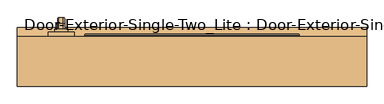
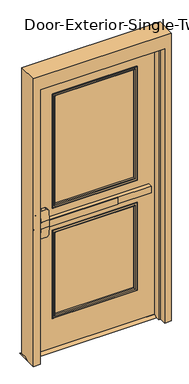
"""IFC4 building model written with IfcOpenShell, lengths in millimetres: door geometry, Door-Exterior-Single-Two_Lite : Door-Exterior-Single-Two_Lite."""

from ifc_helpers import new_model, si_unit, point, frame, frame_2d, origin, place, context, project, spatial, polyline, circle_curve, ellipse_curve, trimmed, segment, composite_curve, outline, extrude, faceted_brep, source, transform, mapped, element, save
from ifc_brep_helpers import plane_surface, cylinder_surface, revolved_surface, advanced_brep


def door_exterior_single_two_lite_door_exterior_single_two_lite_fa13afaf(model_context):
    return source(origin(), model_context, "Body", "SolidModel", [
        extrude(outline(polyline([(44.0, 12.7), (88.45, 12.7), (113.85, 0.0), (18.6, 0.0), (44.0, 12.7)])), frame((-508.0, 0.0, 0.0), z_axis=(1.0, 0.0, 0.0), x_axis=(0.0, 1.0, 0.0)), (0.0, 0.0, 1.0), 1016.0),
        extrude(outline(polyline([(150.2833333, 5.9), (-349.25, 5.9), (-349.25, 12.25), (150.2833333, 12.25), (150.2833333, 5.9)])), frame((0.0, 0.0, 990.6), z_axis=(0.0, 0.0, 1.0), x_axis=(1.0, 0.0, 0.0)), (0.0, 0.0, 1.0), 50.8),
        advanced_brep(
        [(-412.75, 12.25, 1041.4), (-412.75, 12.25, 990.6), (-349.25, 12.25, 990.6), (400.05, 12.25, 990.6), (400.05, 12.25, 1041.4), (-349.25, 12.25, 1041.4), (400.05, 44.0, 1041.4), (400.05, 44.0, 990.6), (-349.25, 44.0, 990.6), (-349.25, 44.0, 927.1), (-368.3, 44.0, 908.05), (-393.7, 44.0, 908.05), (-412.75, 44.0, 927.1), (-412.75, 44.0, 1104.9), (-393.7, 44.0, 1123.95), (-368.3, 44.0, 1123.95), (-349.25, 44.0, 1104.9), (-349.25, 44.0, 1041.4), (-349.25, 15.4252467, 1041.4), (-412.75, 15.4252467, 1041.4), (-412.75, 20.4354269, 1104.9), (-412.75, 20.4354269, 927.1), (-412.75, 15.4252467, 990.6), (-349.25, 15.4252467, 990.6), (-349.25, 20.4354269, 927.1), (-349.25, 20.4354269, 1104.9), (-393.7, 21.938481, 1123.95), (-368.3, 21.938481, 1123.95), (-368.3, 21.938481, 908.05), (-393.7, 21.938481, 908.05)],
        [
            (0, 1),
            (1, 2),
            (2, 3),
            (3, 4),
            (4, 5),
            (5, 0),
            (6, 7),
            (7, 8),
            (8, 9),
            (9, 10, circle_curve(frame((-368.3, 44.0, 927.1), z_axis=(0.0, 1.0, 0.0), x_axis=(1.0, 0.0, 0.0)), 19.05)),
            (10, 11),
            (11, 12, circle_curve(frame((-393.7, 44.0, 927.1), z_axis=(0.0, 1.0, 0.0), x_axis=(1.0, 0.0, 0.0)), 19.05)),
            (12, 13),
            (13, 14, circle_curve(frame((-393.7, 44.0, 1104.9), z_axis=(0.0, 1.0, 0.0), x_axis=(1.0, 0.0, 0.0)), 19.05)),
            (14, 15),
            (15, 16, circle_curve(frame((-368.3, 44.0, 1104.9), z_axis=(0.0, 1.0, 0.0), x_axis=(1.0, 0.0, 0.0)), 19.05)),
            (16, 17),
            (17, 6),
            (4, 6),
            (17, 18),
            (18, 19),
            (19, 0),
            (19, 20),
            (20, 13),
            (12, 21),
            (21, 22),
            (22, 1),
            (7, 3),
            (22, 23),
            (23, 8),
            (23, 24),
            (24, 9),
            (16, 25),
            (25, 18),
            (14, 26),
            (26, 27),
            (27, 15),
            (10, 28),
            (28, 29),
            (29, 11),
            (24, 28, ellipse_curve(frame((-368.3, 20.4354269, 927.1), z_axis=(0.0, 0.9969018152893365, 0.07865602756830282), x_axis=(0.0, -0.07865602756830208, 0.9969018152893365)), 19.1092038, 19.05)),
            (27, 25, ellipse_curve(frame((-368.3, 20.4354269, 1104.9), z_axis=(0.0, 0.9969018152893376, -0.07865602756828934), x_axis=(0.0, -0.078656027568288, -0.9969018152893377)), 19.1092038, 19.05)),
            (20, 26, ellipse_curve(frame((-393.7, 20.4354269, 1104.9), z_axis=(0.0, 0.9969018152893376, -0.07865602756828934), x_axis=(0.0, -0.078656027568288, -0.9969018152893377)), 19.1092038, 19.05)),
            (29, 21, ellipse_curve(frame((-393.7, 20.4354269, 927.1), z_axis=(0.0, 0.9969018152893365, 0.07865602756830282), x_axis=(0.0, -0.07865602756830208, 0.9969018152893365)), 19.1092038, 19.05)),
        ],
        [
            plane_surface(frame((-412.75, 12.25, 1041.4), z_axis=(0.0, -1.0, 0.0), x_axis=(-1.0, 0.0, 0.0))),
            plane_surface(frame((-412.75, 44.0, 1041.4), z_axis=(0.0, 1.0, 0.0), x_axis=(1.0, 0.0, 0.0))),
            plane_surface(frame((400.05, 12.25, 1041.4), z_axis=(0.0, 0.0, 1.0), x_axis=(0.0, 1.0, 0.0))),
            plane_surface(frame((-412.75, 12.25, 1041.4), z_axis=(-1.0, 0.0, 0.0), x_axis=(0.0, 1.0, 0.0))),
            plane_surface(frame((-412.75, 12.25, 990.6), z_axis=(0.0, 0.0, -1.0), x_axis=(0.0, 1.0, 0.0))),
            plane_surface(frame((400.05, 12.25, 990.6), z_axis=(1.0, 0.0, 0.0), x_axis=(0.0, 1.0, 0.0))),
            plane_surface(frame((-349.25, 15.4252467, 927.1), z_axis=(1.0, 0.0, 0.0), x_axis=(0.0, 1.0, 0.0))),
            plane_surface(frame((-368.3, 15.4252467, 1123.95), z_axis=(0.0, 0.0, 1.0), x_axis=(0.0, 1.0, 0.0))),
            plane_surface(frame((-393.7, 15.4252467, 908.05), z_axis=(0.0, 0.0, -1.0), x_axis=(0.0, 1.0, 0.0))),
            cylinder_surface(frame((-368.3, 44.0, 927.1), z_axis=(0.0, -1.0, 0.0), x_axis=(1.0, 0.0, 0.0)), 19.05),
            cylinder_surface(frame((-368.3, 44.0, 1104.9), z_axis=(0.0, -1.0, 0.0), x_axis=(1.0, 0.0, 0.0)), 19.05),
            cylinder_surface(frame((-393.7, 44.0, 1104.9), z_axis=(0.0, -1.0, 0.0), x_axis=(1.0, 0.0, 0.0)), 19.05),
            cylinder_surface(frame((-393.7, 44.0, 927.1), z_axis=(0.0, -1.0, 0.0), x_axis=(1.0, 0.0, 0.0)), 19.05),
            plane_surface(frame((-349.25, 15.4252467, 1041.4), z_axis=(0.0, -0.9969018152893376, 0.07865602756828934), x_axis=(-1.0, 0.0, 0.0))),
            plane_surface(frame((-349.25, 21.938481, 908.05), z_axis=(0.0, -0.9969018152893365, -0.07865602756830282), x_axis=(-1.0, 0.0, 0.0))),
        ],
        [
            (0, [[1, 2, 3, 4, 5, 6]]),
            (1, [[7, 8, 9, 10, 11, 12, 13, 14, 15, 16, 17, 18]]),
            (2, [[19, -18, 20, 21, 22, -6, -5]]),
            (3, [[-1, -22, 23, 24, -13, 25, 26, 27]]),
            (4, [[28, -3, -2, -27, 29, 30, -8]]),
            (5, [[-4, -28, -7, -19]]),
            (6, [[-9, -30, 31, 32]]),
            (6, [[-17, 33, 34, -20]]),
            (7, [[-15, 35, 36, 37]]),
            (8, [[-11, 38, 39, 40]]),
            (9, [[-10, -32, 41, -38]]),
            (10, [[-16, -37, 42, -33]]),
            (11, [[-14, -24, 43, -35]]),
            (12, [[-12, -40, 44, -25]]),
            (13, [[-21, -34, -42, -36, -43, -23]]),
            (14, [[-26, -44, -39, -41, -31, -29]]),
        ],
    ),
        advanced_brep(
        [(-391.0, 101.15, 1017.190625), (-391.0, 101.15, 1014.809375), (-387.428125, 101.15, 1011.2375), (-374.5715406, 101.15, 1011.2375), (-371.0, 101.15, 1014.8090406), (-371.0, 101.15, 1017.190625), (-374.571875, 101.15, 1020.7625), (-387.428125, 101.15, 1020.7625), (-391.0, 101.15, 887.809375), (-387.428125, 101.15, 884.2375), (-374.571875, 101.15, 884.2375), (-371.0, 101.15, 887.809375), (-371.0, 101.15, 890.1909594), (-374.5715406, 101.15, 893.7625), (-387.428125, 101.15, 893.7625), (-391.0, 101.15, 890.190625), (-391.0, 126.55, 1017.190625), (-391.0, 140.440625, 1003.3), (-391.0, 140.440625, 901.7), (-391.0, 126.55, 887.809375), (-391.0, 126.55, 890.190625), (-391.0, 138.059375, 901.7), (-391.0, 138.059375, 1003.3), (-391.0, 126.55, 1014.809375), (-387.428125, 126.55, 1011.2375), (-374.5715406, 126.55, 1011.2375), (-371.0, 126.55, 1014.8090406), (-371.0, 138.0590406, 1003.3), (-371.0, 138.0590406, 901.7), (-371.0, 126.55, 890.1909594), (-371.0, 126.55, 887.809375), (-371.0, 140.440625, 901.7), (-371.0, 140.440625, 1003.3), (-371.0, 126.55, 1017.190625), (-374.571875, 126.55, 1020.7625), (-387.428125, 126.55, 1020.7625), (-387.428125, 134.4875, 1003.3), (-374.5715406, 134.4875, 1003.3), (-374.571875, 144.0125, 1003.3), (-387.428125, 144.0125, 1003.3), (-387.428125, 134.4875, 901.7), (-374.5715406, 134.4875, 901.7), (-374.571875, 144.0125, 901.7), (-387.428125, 144.0125, 901.7), (-387.428125, 126.55, 893.7625), (-374.5715406, 126.55, 893.7625), (-374.571875, 126.55, 884.2375), (-387.428125, 126.55, 884.2375)],
        [
            (0, 1),
            (1, 2, circle_curve(frame((-387.428125, 101.15, 1014.809375), z_axis=(0.0, -1.0, 0.0), x_axis=(0.0, 0.0, 1.0)), 3.571875)),
            (2, 3),
            (3, 4, circle_curve(frame((-374.5715406, 101.15, 1014.8090406), z_axis=(0.0, -1.0, 0.0), x_axis=(0.0, 0.0, 1.0)), 3.5715406)),
            (4, 5),
            (5, 6, circle_curve(frame((-374.571875, 101.15, 1017.190625), z_axis=(0.0, -1.0, 0.0), x_axis=(0.0, 0.0, 1.0)), 3.571875)),
            (6, 7),
            (7, 0, circle_curve(frame((-387.428125, 101.15, 1017.190625), z_axis=(0.0, -1.0, 0.0), x_axis=(0.0, 0.0, 1.0)), 3.571875)),
            (8, 9, circle_curve(frame((-387.428125, 101.15, 887.809375), z_axis=(0.0, -1.0, 0.0), x_axis=(0.0, 0.0, -1.0)), 3.571875)),
            (9, 10),
            (10, 11, circle_curve(frame((-374.571875, 101.15, 887.809375), z_axis=(0.0, -1.0, 0.0), x_axis=(0.0, 0.0, -1.0)), 3.571875)),
            (11, 12),
            (12, 13, circle_curve(frame((-374.5715406, 101.15, 890.1909594), z_axis=(0.0, -1.0, 0.0), x_axis=(0.0, 0.0, -1.0)), 3.5715406)),
            (13, 14),
            (14, 15, circle_curve(frame((-387.428125, 101.15, 890.190625), z_axis=(0.0, -1.0, 0.0), x_axis=(0.0, 0.0, -1.0)), 3.571875)),
            (15, 8),
            (0, 16),
            (16, 17, circle_curve(frame((-391.0, 126.55, 1003.3), z_axis=(-1.0, 0.0, 0.0), x_axis=(0.0, 0.0, 1.0)), 13.890625)),
            (17, 18),
            (18, 19, circle_curve(frame((-391.0, 126.55, 901.7), z_axis=(-1.0, 0.0, 0.0), x_axis=(0.0, 1.0, 0.0)), 13.890625)),
            (19, 8),
            (15, 20),
            (20, 21, circle_curve(frame((-391.0, 126.55, 901.7), z_axis=(1.0, 0.0, 0.0), x_axis=(0.0, 1.0, 0.0)), 11.509375)),
            (21, 22),
            (22, 23, circle_curve(frame((-391.0, 126.55, 1003.3), z_axis=(1.0, 0.0, 0.0), x_axis=(0.0, 0.0, 1.0)), 11.509375)),
            (23, 1),
            (23, 24, circle_curve(frame((-387.428125, 126.55, 1014.809375), z_axis=(0.0, -1.0, 0.0), x_axis=(0.0, 0.0, 1.0)), 3.571875)),
            (24, 2),
            (24, 25),
            (25, 3),
            (25, 26, circle_curve(frame((-374.5715406, 126.55, 1014.8090406), z_axis=(0.0, -1.0, 0.0), x_axis=(0.0, 0.0, 1.0)), 3.5715406)),
            (26, 4),
            (26, 27, circle_curve(frame((-371.0, 126.55, 1003.3), z_axis=(-1.0, 0.0, 0.0), x_axis=(0.0, 0.0, 1.0)), 11.5090406)),
            (27, 28),
            (28, 29, circle_curve(frame((-371.0, 126.55, 901.7), z_axis=(-1.0, 0.0, 0.0), x_axis=(0.0, 1.0, 0.0)), 11.5090406)),
            (29, 12),
            (11, 30),
            (30, 31, circle_curve(frame((-371.0, 126.55, 901.7), z_axis=(1.0, 0.0, 0.0), x_axis=(0.0, 1.0, 0.0)), 13.890625)),
            (31, 32),
            (32, 33, circle_curve(frame((-371.0, 126.55, 1003.3), z_axis=(1.0, 0.0, 0.0), x_axis=(0.0, 0.0, 1.0)), 13.890625)),
            (33, 5),
            (33, 34, circle_curve(frame((-374.571875, 126.55, 1017.190625), z_axis=(0.0, -1.0, 0.0), x_axis=(0.0, 0.0, 1.0)), 3.571875)),
            (34, 6),
            (34, 35),
            (35, 7),
            (35, 16, circle_curve(frame((-387.428125, 126.55, 1017.190625), z_axis=(0.0, -1.0, 0.0), x_axis=(0.0, 0.0, 1.0)), 3.571875)),
            (36, 24, circle_curve(frame((-387.428125, 126.55, 1003.3), z_axis=(1.0, 0.0, 0.0), x_axis=(0.0, 0.0, 1.0)), 7.9375)),
            (22, 36, circle_curve(frame((-387.428125, 138.059375, 1003.3), z_axis=(0.0, 0.0, 1.0), x_axis=(0.0, 1.0, 0.0)), 3.571875)),
            (37, 25, circle_curve(frame((-374.5715406, 126.55, 1003.3), z_axis=(1.0, 0.0, 0.0), x_axis=(0.0, 0.0, 1.0)), 7.9375)),
            (36, 37),
            (37, 27, circle_curve(frame((-374.5715406, 138.0590406, 1003.3), z_axis=(0.0, 0.0, 1.0), x_axis=(0.0, 1.0, 0.0)), 3.5715406)),
            (38, 34, circle_curve(frame((-374.571875, 126.55, 1003.3), z_axis=(1.0, 0.0, 0.0), x_axis=(0.0, 0.0, 1.0)), 17.4625)),
            (32, 38, circle_curve(frame((-374.571875, 140.440625, 1003.3), z_axis=(0.0, 0.0, 1.0), x_axis=(0.0, 1.0, 0.0)), 3.571875)),
            (39, 35, circle_curve(frame((-387.428125, 126.55, 1003.3), z_axis=(1.0, 0.0, 0.0), x_axis=(0.0, 0.0, 1.0)), 17.4625)),
            (38, 39),
            (39, 17, circle_curve(frame((-387.428125, 140.440625, 1003.3), z_axis=(0.0, 0.0, 1.0), x_axis=(0.0, 1.0, 0.0)), 3.571875)),
            (21, 40, circle_curve(frame((-387.428125, 138.059375, 901.7), z_axis=(0.0, 0.0, 1.0), x_axis=(0.0, 1.0, 0.0)), 3.571875)),
            (40, 36),
            (40, 41),
            (41, 37),
            (41, 28, circle_curve(frame((-374.5715406, 138.0590406, 901.7), z_axis=(0.0, 0.0, 1.0), x_axis=(0.0, 1.0, 0.0)), 3.5715406)),
            (31, 42, circle_curve(frame((-374.571875, 140.440625, 901.7), z_axis=(0.0, 0.0, 1.0), x_axis=(0.0, 1.0, 0.0)), 3.571875)),
            (42, 38),
            (42, 43),
            (43, 39),
            (43, 18, circle_curve(frame((-387.428125, 140.440625, 901.7), z_axis=(0.0, 0.0, 1.0), x_axis=(0.0, 1.0, 0.0)), 3.571875)),
            (44, 40, circle_curve(frame((-387.428125, 126.55, 901.7), z_axis=(1.0, 0.0, 0.0), x_axis=(0.0, 1.0, 0.0)), 7.9375)),
            (20, 44, circle_curve(frame((-387.428125, 126.55, 890.190625), z_axis=(0.0, 1.0, 0.0), x_axis=(0.0, 0.0, -1.0)), 3.571875)),
            (45, 41, circle_curve(frame((-374.5715406, 126.55, 901.7), z_axis=(1.0, 0.0, 0.0), x_axis=(0.0, 1.0, 0.0)), 7.9375)),
            (44, 45),
            (45, 29, circle_curve(frame((-374.5715406, 126.55, 890.1909594), z_axis=(0.0, 1.0, 0.0), x_axis=(0.0, 0.0, -1.0)), 3.5715406)),
            (46, 42, circle_curve(frame((-374.571875, 126.55, 901.7), z_axis=(1.0, 0.0, 0.0), x_axis=(0.0, 1.0, 0.0)), 17.4625)),
            (30, 46, circle_curve(frame((-374.571875, 126.55, 887.809375), z_axis=(0.0, 1.0, 0.0), x_axis=(0.0, 0.0, -1.0)), 3.571875)),
            (47, 43, circle_curve(frame((-387.428125, 126.55, 901.7), z_axis=(1.0, 0.0, 0.0), x_axis=(0.0, 1.0, 0.0)), 17.4625)),
            (46, 47),
            (47, 19, circle_curve(frame((-387.428125, 126.55, 887.809375), z_axis=(0.0, 1.0, 0.0), x_axis=(0.0, 0.0, -1.0)), 3.571875)),
            (14, 44),
            (13, 45),
            (10, 46),
            (9, 47),
        ],
        [
            plane_surface(frame((-381.0, 101.15, 1016.0), z_axis=(0.0, -1.0, 0.0), x_axis=(1.0, 0.0, 0.0))),
            plane_surface(frame((-381.0, 101.15, 889.0), z_axis=(0.0, -1.0, 0.0), x_axis=(1.0, 0.0, 0.0))),
            plane_surface(frame((-391.0, 101.15, 1017.190625), z_axis=(-1.0, 0.0, 0.0), x_axis=(0.0, 1.0, 0.0))),
            cylinder_surface(frame((-387.428125, 101.15, 1014.809375), z_axis=(0.0, -1.0, 0.0), x_axis=(0.0, 0.0, 1.0)), 3.571875),
            plane_surface(frame((-387.428125, 101.15, 1011.2375), z_axis=(0.0, 0.0, -1.0), x_axis=(0.0, 1.0, 0.0))),
            cylinder_surface(frame((-374.5715406, 101.15, 1014.8090406), z_axis=(0.0, -1.0, 0.0), x_axis=(0.0, 0.0, 1.0)), 3.5715406),
            plane_surface(frame((-371.0, 101.15, 1014.8090406), z_axis=(1.0, 0.0, 0.0), x_axis=(0.0, 1.0, 0.0))),
            cylinder_surface(frame((-374.571875, 101.15, 1017.190625), z_axis=(0.0, -1.0, 0.0), x_axis=(0.0, 0.0, 1.0)), 3.571875),
            plane_surface(frame((-374.571875, 101.15, 1020.7625), z_axis=(0.0, 0.0, 1.0), x_axis=(0.0, 1.0, 0.0))),
            cylinder_surface(frame((-387.428125, 101.15, 1017.190625), z_axis=(0.0, -1.0, 0.0), x_axis=(0.0, 0.0, 1.0)), 3.571875),
            revolved_surface(trimmed(ellipse_curve(frame((-387.428125, 126.55, 1014.809375), z_axis=(0.0, -1.0, 0.0), x_axis=(0.0, 0.0, 1.0)), 3.571875, 3.571875), [point((-391.0, 126.55, 1014.809375))], [point((-387.428125, 126.55, 1011.2375))], True, "CARTESIAN"), (-381.0, 126.55, 1003.3), (-1.0, 0.0, 0.0)),
            revolved_surface(polyline([(-387.428125, 126.55, 1011.2375), (-374.5715406, 126.55, 1011.2375)]), (-381.0, 126.55, 1003.3), (-1.0, 0.0, 0.0)),
            revolved_surface(trimmed(ellipse_curve(frame((-374.5715406, 126.55, 1014.8090406), z_axis=(0.0, -1.0, 0.0), x_axis=(0.0, 0.0, 1.0)), 3.5715406, 3.5715406), [point((-374.5715406, 126.55, 1011.2375))], [point((-371.0, 126.55, 1014.8090406))], True, "CARTESIAN"), (-381.0, 126.55, 1003.3), (-1.0, 0.0, 0.0)),
            revolved_surface(trimmed(ellipse_curve(frame((-374.571875, 126.55, 1017.190625), z_axis=(0.0, -1.0, 0.0), x_axis=(0.0, 0.0, 1.0)), 3.571875, 3.571875), [point((-371.0, 126.55, 1017.190625))], [point((-374.571875, 126.55, 1020.7625))], True, "CARTESIAN"), (-381.0, 126.55, 1003.3), (-1.0, 0.0, 0.0)),
            cylinder_surface(frame((-381.0, 126.55, 1003.3), z_axis=(-1.0, 0.0, 0.0), x_axis=(0.0, 0.0, 1.0)), 17.4625),
            revolved_surface(trimmed(ellipse_curve(frame((-387.428125, 126.55, 1017.190625), z_axis=(0.0, -1.0, 0.0), x_axis=(0.0, 0.0, 1.0)), 3.571875, 3.571875), [point((-387.428125, 126.55, 1020.7625))], [point((-391.0, 126.55, 1017.190625))], True, "CARTESIAN"), (-381.0, 126.55, 1003.3), (-1.0, 0.0, 0.0)),
            cylinder_surface(frame((-387.428125, 138.059375, 1003.3), z_axis=(0.0, 0.0, 1.0), x_axis=(0.0, 1.0, 0.0)), 3.571875),
            plane_surface(frame((-387.428125, 134.4875, 1003.3), z_axis=(0.0, -1.0, 0.0), x_axis=(0.0, 0.0, -1.0))),
            cylinder_surface(frame((-374.5715406, 138.0590406, 1003.3), z_axis=(0.0, 0.0, 1.0), x_axis=(0.0, 1.0, 0.0)), 3.5715406),
            cylinder_surface(frame((-374.571875, 140.440625, 1003.3), z_axis=(0.0, 0.0, 1.0), x_axis=(0.0, 1.0, 0.0)), 3.571875),
            plane_surface(frame((-374.571875, 144.0125, 1003.3), z_axis=(0.0, 1.0, 0.0), x_axis=(0.0, 0.0, -1.0))),
            cylinder_surface(frame((-387.428125, 140.440625, 1003.3), z_axis=(0.0, 0.0, 1.0), x_axis=(0.0, 1.0, 0.0)), 3.571875),
            revolved_surface(trimmed(ellipse_curve(frame((-387.428125, 138.059375, 901.7), z_axis=(0.0, 0.0, 1.0), x_axis=(0.0, 1.0, 0.0)), 3.571875, 3.571875), [point((-391.0, 138.059375, 901.7))], [point((-387.428125, 134.4875, 901.7))], True, "CARTESIAN"), (-381.0, 126.55, 901.7), (-1.0, 0.0, 0.0)),
            revolved_surface(polyline([(-387.428125, 134.4875, 901.7), (-374.5715406, 134.4875, 901.7)]), (-381.0, 126.55, 901.7), (-1.0, 0.0, 0.0)),
            revolved_surface(trimmed(ellipse_curve(frame((-374.5715406, 138.0590406, 901.7), z_axis=(0.0, 0.0, 1.0), x_axis=(0.0, 1.0, 0.0)), 3.5715406, 3.5715406), [point((-374.5715406, 134.4875, 901.7))], [point((-371.0, 138.0590406, 901.7))], True, "CARTESIAN"), (-381.0, 126.55, 901.7), (-1.0, 0.0, 0.0)),
            revolved_surface(trimmed(ellipse_curve(frame((-374.571875, 140.440625, 901.7), z_axis=(0.0, 0.0, 1.0), x_axis=(0.0, 1.0, 0.0)), 3.571875, 3.571875), [point((-371.0, 140.440625, 901.7))], [point((-374.571875, 144.0125, 901.7))], True, "CARTESIAN"), (-381.0, 126.55, 901.7), (-1.0, 0.0, 0.0)),
            cylinder_surface(frame((-381.0, 126.55, 901.7), z_axis=(-1.0, 0.0, 0.0), x_axis=(0.0, 1.0, 0.0)), 17.4625),
            revolved_surface(trimmed(ellipse_curve(frame((-387.428125, 140.440625, 901.7), z_axis=(0.0, 0.0, 1.0), x_axis=(0.0, 1.0, 0.0)), 3.571875, 3.571875), [point((-387.428125, 144.0125, 901.7))], [point((-391.0, 140.440625, 901.7))], True, "CARTESIAN"), (-381.0, 126.55, 901.7), (-1.0, 0.0, 0.0)),
            cylinder_surface(frame((-387.428125, 126.55, 890.190625), z_axis=(0.0, 1.0, 0.0), x_axis=(0.0, 0.0, -1.0)), 3.571875),
            plane_surface(frame((-387.428125, 126.55, 893.7625), z_axis=(0.0, 0.0, 1.0), x_axis=(0.0, -1.0, 0.0))),
            cylinder_surface(frame((-374.5715406, 126.55, 890.1909594), z_axis=(0.0, 1.0, 0.0), x_axis=(0.0, 0.0, -1.0)), 3.5715406),
            cylinder_surface(frame((-374.571875, 126.55, 887.809375), z_axis=(0.0, 1.0, 0.0), x_axis=(0.0, 0.0, -1.0)), 3.571875),
            plane_surface(frame((-374.571875, 126.55, 884.2375), z_axis=(0.0, 0.0, -1.0), x_axis=(0.0, -1.0, 0.0))),
            cylinder_surface(frame((-387.428125, 126.55, 887.809375), z_axis=(0.0, 1.0, 0.0), x_axis=(0.0, 0.0, -1.0)), 3.571875),
        ],
        [
            (0, [[1, 2, 3, 4, 5, 6, 7, 8]]),
            (1, [[9, 10, 11, 12, 13, 14, 15, 16]]),
            (2, [[-1, 17, 18, 19, 20, 21, -16, 22, 23, 24, 25, 26]]),
            (3, [[-2, -26, 27, 28]]),
            (4, [[-3, -28, 29, 30]]),
            (5, [[-4, -30, 31, 32]]),
            (6, [[-5, -32, 33, 34, 35, 36, -12, 37, 38, 39, 40, 41]]),
            (7, [[-6, -41, 42, 43]]),
            (8, [[-7, -43, 44, 45]]),
            (9, [[-8, -45, 46, -17]]),
            (10, [[47, -27, -25, 48]]),
            (11, [[49, -29, -47, 50]]),
            (12, [[-33, -31, -49, 51]]),
            (13, [[52, -42, -40, 53]]),
            (14, [[54, -44, -52, 55]]),
            (15, [[-18, -46, -54, 56]]),
            (16, [[-48, -24, 57, 58]]),
            (17, [[-50, -58, 59, 60]]),
            (18, [[-51, -60, 61, -34]]),
            (19, [[-53, -39, 62, 63]]),
            (20, [[-55, -63, 64, 65]]),
            (21, [[-56, -65, 66, -19]]),
            (22, [[67, -57, -23, 68]]),
            (23, [[69, -59, -67, 70]]),
            (24, [[-35, -61, -69, 71]]),
            (25, [[72, -62, -38, 73]]),
            (26, [[74, -64, -72, 75]]),
            (27, [[-20, -66, -74, 76]]),
            (28, [[-68, -22, -15, 77]]),
            (29, [[-70, -77, -14, 78]]),
            (30, [[-71, -78, -13, -36]]),
            (31, [[-73, -37, -11, 79]]),
            (32, [[-75, -79, -10, 80]]),
            (33, [[-76, -80, -9, -21]]),
        ],
    ),
        extrude(outline(composite_curve([segment(trimmed(circle_curve(frame_2d((1117.6, -381.0)), 19.0), [point((1117.6, -400.0))], [point((1117.6, -362.0))], False, "CARTESIAN"), True, "CONTINUOUS"), segment(trimmed(circle_curve(frame_2d((1117.6, -381.0)), 19.0), [point((1117.6, -362.0))], [point((1117.6, -400.0))], False, "CARTESIAN"), True, "CONTINUOUS")], self_intersect=False)), frame((0.0, 101.15, 0.0), z_axis=(0.0, 1.0, 0.0), x_axis=(0.0, 0.0, 1.0)), (0.0, 0.0, 1.0), 8.73125),
        extrude(outline(composite_curve([segment(trimmed(circle_curve(frame_2d((1113.0338574, -381.0)), 89.3016225), [point((1193.8, -342.9))], [point((1193.8, -419.1))], False, "CARTESIAN"), True, "CONTINUOUS"), segment(polyline([(1193.8, -419.1), (838.2, -419.1)]), True, "CONTINUOUS"), segment(trimmed(circle_curve(frame_2d((918.9661426, -381.0)), 89.3016225), [point((838.2, -419.1))], [point((838.2, -342.9))], False, "CARTESIAN"), True, "CONTINUOUS"), segment(polyline([(838.2, -342.9), (1193.8, -342.9)]), True, "CONTINUOUS")], self_intersect=False)), frame((0.0, 88.45, 0.0), z_axis=(0.0, 1.0, 0.0), x_axis=(0.0, 0.0, 1.0)), (0.0, 0.0, 1.0), 12.7),
        extrude(outline(polyline([(2133.6, -457.2), (12.7, -457.2), (12.7, 457.2), (2133.6, 457.2), (2133.6, -457.2)]), holes=[polyline([(1981.2, -304.8), (1981.2, 304.8), (1111.25, 304.8), (1111.25, -304.8), (1981.2, -304.8)]), polyline([(920.75, -304.8), (920.75, 304.8), (254.0, 304.8), (254.0, -304.8), (920.75, -304.8)])]), frame((0.0, 44.0, 0.0), z_axis=(0.0, 1.0, 0.0), x_axis=(0.0, 0.0, 1.0)), (0.0, 0.0, 1.0), 44.45),
        faceted_brep([(457.2, 39.2375, 0.0), (457.2, 88.45, 0.0), (508.0, 88.45, 0.0), (508.0, -57.6, 0.0), (457.2, -57.6, 0.0), (457.2, -8.3875, 0.0), (441.325, -8.3875, 0.0), (441.325, 39.2375, 0.0), (457.2, 39.2375, 2133.6), (457.2, 88.45, 2133.6), (-457.2, 88.45, 2133.6), (-457.2, 88.45, 0.0), (-508.0, 88.45, 0.0), (-508.0, 88.45, 2235.2), (508.0, 88.45, 2235.2), (508.0, -57.6, 2235.2), (-508.0, -57.6, 2235.2), (-508.0, -57.6, 0.0), (-457.2, -57.6, 0.0), (-457.2, -57.6, 2133.6), (457.2, -57.6, 2133.6), (457.2, -8.3875, 2133.6), (-457.2, -8.3875, 2133.6), (-457.2, -8.3875, 0.0), (-441.325, -8.3875, 0.0), (-441.325, -8.3875, 2117.725), (441.325, -8.3875, 2117.725), (441.325, 39.2375, 2117.725), (-441.325, 39.2375, 2117.725), (-441.325, 39.2375, 0.0), (-457.2, 39.2375, 0.0), (-457.2, 39.2375, 2133.6)], [[[0, 1, 2, 3, 4, 5, 6, 7]], [[1, 0, 8, 9]], [[2, 1, 9, 10, 11, 12, 13, 14]], [[3, 2, 14, 15]], [[4, 3, 15, 16, 17, 18, 19, 20]], [[5, 4, 20, 21]], [[6, 5, 21, 22, 23, 24, 25, 26]], [[7, 6, 26, 27]], [[0, 7, 27, 28, 29, 30, 31, 8]], [[9, 8, 31, 10]], [[20, 19, 22, 21]], [[26, 25, 28, 27]], [[12, 11, 30, 29, 24, 23, 18, 17]], [[11, 10, 31, 30]], [[13, 12, 17, 16]], [[19, 18, 23, 22]], [[25, 24, 29, 28]], [[15, 14, 13, 16]]]),
        extrude(outline(polyline([(304.8, 56.7), (-304.8, 56.7), (-304.8, 75.75), (304.8, 75.75), (304.8, 56.7)])), frame((0.0, 0.0, 1111.25), z_axis=(0.0, 0.0, 1.0), x_axis=(1.0, 0.0, 0.0)), (0.0, 0.0, 1.0), 869.95),
        extrude(outline(polyline([(304.8, 56.7), (-304.8, 56.7), (-304.8, 75.75), (304.8, 75.75), (304.8, 56.7)])), frame((0.0, 0.0, 254.0), z_axis=(0.0, 0.0, 1.0), x_axis=(1.0, 0.0, 0.0)), (0.0, 0.0, 1.0), 666.75),
        advanced_brep(
        [(-304.8, 75.75, 1981.2), (-304.8, 88.45, 1981.2), (-304.8, 88.45, 1111.25), (-304.8, 75.75, 1111.25), (-292.8, 89.45, 1969.2), (-292.8, 75.75, 1969.2), (-292.8, 75.75, 1123.25), (-292.8, 89.45, 1123.25), (-297.8, 94.45, 1974.2), (-297.8, 94.45, 1118.25), (-312.8, 92.45, 1989.2), (-310.8, 94.45, 1987.2), (-310.8, 94.45, 1105.25), (-312.8, 92.45, 1103.25), (-312.8, 88.45, 1989.2), (-312.8, 88.45, 1103.25), (304.8, 88.45, 1111.25), (304.8, 75.75, 1111.25), (292.8, 75.75, 1123.25), (292.8, 89.45, 1123.25), (297.8, 94.45, 1118.25), (310.8, 94.45, 1105.25), (312.8, 92.45, 1103.25), (312.8, 88.45, 1103.25), (304.8, 88.45, 1981.2), (304.8, 75.75, 1981.2), (292.8, 75.75, 1969.2), (292.8, 89.45, 1969.2), (297.8, 94.45, 1974.2), (310.8, 94.45, 1987.2), (312.8, 92.45, 1989.2), (312.8, 88.45, 1989.2)],
        [
            (0, 1),
            (1, 2),
            (2, 3),
            (3, 0),
            (4, 5),
            (5, 6),
            (6, 7),
            (7, 4),
            (8, 4, ellipse_curve(frame((-297.8, 89.45, 1974.2), z_axis=(-0.7071067811865475, 0.0, -0.7071067811865475), x_axis=(-0.7071067811865474, 0.0, 0.7071067811865476)), 7.0710678, 5.0)),
            (7, 9, ellipse_curve(frame((-297.8, 89.45, 1118.25), z_axis=(-0.7071067811865475, 0.0, 0.7071067811865475), x_axis=(0.7071067811865474, 0.0, 0.7071067811865476)), 7.0710678, 5.0)),
            (9, 8),
            (10, 11, ellipse_curve(frame((-310.8, 92.45, 1987.2), z_axis=(-0.7071067811865475, 0.0, -0.7071067811865475), x_axis=(-0.7071067811865474, 0.0, 0.7071067811865476)), 2.8284271, 2.0)),
            (11, 12),
            (12, 13, ellipse_curve(frame((-310.8, 92.45, 1105.25), z_axis=(-0.7071067811865475, 0.0, 0.7071067811865475), x_axis=(0.7071067811865474, 0.0, 0.7071067811865476)), 2.8284271, 2.0)),
            (13, 10),
            (14, 10),
            (13, 15),
            (15, 14),
            (2, 16),
            (16, 17),
            (17, 3),
            (6, 18),
            (18, 19),
            (19, 7),
            (19, 20, ellipse_curve(frame((297.8, 89.45, 1118.25), z_axis=(-0.7071067811865475, 0.0, -0.7071067811865475), x_axis=(-0.7071067811865476, 0.0, 0.7071067811865474)), 7.0710678, 5.0)),
            (20, 9),
            (12, 21),
            (21, 22, ellipse_curve(frame((310.8, 92.45, 1105.25), z_axis=(-0.7071067811865475, 0.0, -0.7071067811865475), x_axis=(-0.7071067811865476, 0.0, 0.7071067811865474)), 2.8284271, 2.0)),
            (22, 13),
            (22, 23),
            (23, 15),
            (16, 24),
            (24, 25),
            (25, 17),
            (18, 26),
            (26, 27),
            (27, 19),
            (27, 28, ellipse_curve(frame((297.8, 89.45, 1974.2), z_axis=(0.7071067811865475, 0.0, -0.7071067811865475), x_axis=(-0.7071067811865474, 0.0, -0.7071067811865476)), 7.0710678, 5.0)),
            (28, 20),
            (21, 29),
            (29, 30, ellipse_curve(frame((310.8, 92.45, 1987.2), z_axis=(0.7071067811865475, 0.0, -0.7071067811865475), x_axis=(-0.7071067811865474, 0.0, -0.7071067811865476)), 2.8284271, 2.0)),
            (30, 22),
            (30, 31),
            (31, 23),
            (31, 14),
            (1, 24),
            (0, 25),
            (5, 26),
            (4, 27),
            (8, 28),
            (11, 29),
            (10, 30),
        ],
        [
            plane_surface(frame((-304.8, 88.45, 1981.2), z_axis=(-1.0, 0.0, 0.0), x_axis=(0.0, 0.0, -1.0))),
            plane_surface(frame((-292.8, 75.75, 1969.2), z_axis=(1.0, 0.0, 0.0), x_axis=(0.0, 0.0, -1.0))),
            cylinder_surface(frame((-297.8, 89.45, 1981.2), z_axis=(0.0, 0.0, 1.0), x_axis=(-1.0, 0.0, 0.0)), 5.0),
            cylinder_surface(frame((-310.8, 92.45, 1981.2), z_axis=(0.0, 0.0, 1.0), x_axis=(-1.0, 0.0, 0.0)), 2.0),
            plane_surface(frame((-312.8, 92.45, 1989.2), z_axis=(-1.0, 0.0, 0.0), x_axis=(0.0, 0.0, -1.0))),
            plane_surface(frame((-304.8, 88.45, 1111.25), z_axis=(0.0, 0.0, -1.0), x_axis=(1.0, 0.0, 0.0))),
            plane_surface(frame((-292.8, 75.75, 1123.25), z_axis=(0.0, 0.0, 1.0), x_axis=(1.0, 0.0, 0.0))),
            cylinder_surface(frame((-304.8, 89.45, 1118.25), z_axis=(-1.0, 0.0, 0.0), x_axis=(0.0, 0.0, -1.0)), 5.0),
            cylinder_surface(frame((-304.8, 92.45, 1105.25), z_axis=(-1.0, 0.0, 0.0), x_axis=(0.0, 0.0, -1.0)), 2.0),
            plane_surface(frame((-312.8, 92.45, 1103.25), z_axis=(0.0, 0.0, -1.0), x_axis=(1.0, 0.0, 0.0))),
            plane_surface(frame((304.8, 88.45, 1111.25), z_axis=(1.0, 0.0, 0.0), x_axis=(0.0, 0.0, 1.0))),
            plane_surface(frame((292.8, 75.75, 1123.25), z_axis=(-1.0, 0.0, 0.0), x_axis=(0.0, 0.0, 1.0))),
            cylinder_surface(frame((297.8, 89.45, 1111.25), z_axis=(0.0, 0.0, -1.0), x_axis=(1.0, 0.0, 0.0)), 5.0),
            cylinder_surface(frame((310.8, 92.45, 1111.25), z_axis=(0.0, 0.0, -1.0), x_axis=(1.0, 0.0, 0.0)), 2.0),
            plane_surface(frame((312.8, 92.45, 1103.25), z_axis=(1.0, 0.0, 0.0), x_axis=(0.0, 0.0, 1.0))),
            plane_surface(frame((312.8, 88.45, 1989.2), z_axis=(0.0, -1.0, 0.0), x_axis=(-1.0, 0.0, 0.0))),
            plane_surface(frame((304.8, 88.45, 1981.2), z_axis=(0.0, 0.0, 1.0), x_axis=(-1.0, 0.0, 0.0))),
            plane_surface(frame((304.8, 75.75, 1981.2), z_axis=(0.0, -1.0, 0.0), x_axis=(-1.0, 0.0, 0.0))),
            plane_surface(frame((292.8, 75.75, 1969.2), z_axis=(0.0, 0.0, -1.0), x_axis=(-1.0, 0.0, 0.0))),
            cylinder_surface(frame((304.8, 89.45, 1974.2), z_axis=(1.0, 0.0, 0.0), x_axis=(0.0, 0.0, 1.0)), 5.0),
            plane_surface(frame((297.8, 94.45, 1974.2), z_axis=(0.0, 1.0, 0.0), x_axis=(-1.0, 0.0, 0.0))),
            cylinder_surface(frame((304.8, 92.45, 1987.2), z_axis=(1.0, 0.0, 0.0), x_axis=(0.0, 0.0, 1.0)), 2.0),
            plane_surface(frame((312.8, 92.45, 1989.2), z_axis=(0.0, 0.0, 1.0), x_axis=(-1.0, 0.0, 0.0))),
        ],
        [
            (0, [[1, 2, 3, 4]]),
            (1, [[5, 6, 7, 8]]),
            (2, [[9, -8, 10, 11]]),
            (3, [[12, 13, 14, 15]]),
            (4, [[16, -15, 17, 18]]),
            (5, [[-3, 19, 20, 21]]),
            (6, [[-7, 22, 23, 24]]),
            (7, [[-10, -24, 25, 26]]),
            (8, [[-14, 27, 28, 29]]),
            (9, [[-17, -29, 30, 31]]),
            (10, [[-20, 32, 33, 34]]),
            (11, [[-23, 35, 36, 37]]),
            (12, [[-25, -37, 38, 39]]),
            (13, [[-28, 40, 41, 42]]),
            (14, [[-30, -42, 43, 44]]),
            (15, [[-31, -44, 45, -18], [46, -32, -19, -2]]),
            (16, [[-33, -46, -1, 47]]),
            (17, [[-21, -34, -47, -4], [48, -35, -22, -6]]),
            (18, [[-36, -48, -5, 49]]),
            (19, [[-38, -49, -9, 50]]),
            (20, [[51, -40, -27, -13], [-26, -39, -50, -11]]),
            (21, [[-41, -51, -12, 52]]),
            (22, [[-43, -52, -16, -45]]),
        ],
    ),
        advanced_brep(
        [(-304.8, 56.7, 1111.25), (-304.8, 44.0, 1111.25), (-304.8, 44.0, 1981.2), (-304.8, 56.7, 1981.2), (-292.8, 43.0, 1123.25), (-292.8, 56.7, 1123.25), (-292.8, 56.7, 1969.2), (-292.8, 43.0, 1969.2), (-297.8, 38.0, 1118.25), (-297.8, 38.0, 1974.2), (-312.8, 40.0, 1103.25), (-310.8, 38.0, 1105.25), (-310.8, 38.0, 1987.2), (-312.8, 40.0, 1989.2), (-312.8, 44.0, 1103.25), (-312.8, 44.0, 1989.2), (304.8, 44.0, 1981.2), (304.8, 56.7, 1981.2), (292.8, 56.7, 1969.2), (292.8, 43.0, 1969.2), (297.8, 38.0, 1974.2), (310.8, 38.0, 1987.2), (312.8, 40.0, 1989.2), (312.8, 44.0, 1989.2), (304.8, 44.0, 1111.25), (304.8, 56.7, 1111.25), (292.8, 56.7, 1123.25), (292.8, 43.0, 1123.25), (297.8, 38.0, 1118.25), (310.8, 38.0, 1105.25), (312.8, 40.0, 1103.25), (312.8, 44.0, 1103.25)],
        [
            (0, 1),
            (1, 2),
            (2, 3),
            (3, 0),
            (4, 5),
            (5, 6),
            (6, 7),
            (7, 4),
            (8, 4, ellipse_curve(frame((-297.8, 43.0, 1118.25), z_axis=(-0.7071067811865475, 0.0, 0.7071067811865475), x_axis=(-0.7071067811865474, 0.0, -0.7071067811865476)), 7.0710678, 5.0)),
            (7, 9, ellipse_curve(frame((-297.8, 43.0, 1974.2), z_axis=(-0.7071067811865475, 0.0, -0.7071067811865475), x_axis=(0.7071067811865474, 0.0, -0.7071067811865476)), 7.0710678, 5.0)),
            (9, 8),
            (10, 11, ellipse_curve(frame((-310.8, 40.0, 1105.25), z_axis=(-0.7071067811865475, 0.0, 0.7071067811865475), x_axis=(-0.7071067811865474, 0.0, -0.7071067811865476)), 2.8284271, 2.0)),
            (11, 12),
            (12, 13, ellipse_curve(frame((-310.8, 40.0, 1987.2), z_axis=(-0.7071067811865475, 0.0, -0.7071067811865475), x_axis=(0.7071067811865474, 0.0, -0.7071067811865476)), 2.8284271, 2.0)),
            (13, 10),
            (14, 10),
            (13, 15),
            (15, 14),
            (2, 16),
            (16, 17),
            (17, 3),
            (6, 18),
            (18, 19),
            (19, 7),
            (19, 20, ellipse_curve(frame((297.8, 43.0, 1974.2), z_axis=(-0.7071067811865475, 0.0, 0.7071067811865475), x_axis=(-0.7071067811865476, 0.0, -0.7071067811865474)), 7.0710678, 5.0)),
            (20, 9),
            (12, 21),
            (21, 22, ellipse_curve(frame((310.8, 40.0, 1987.2), z_axis=(-0.7071067811865475, 0.0, 0.7071067811865475), x_axis=(-0.7071067811865476, 0.0, -0.7071067811865474)), 2.8284271, 2.0)),
            (22, 13),
            (22, 23),
            (23, 15),
            (16, 24),
            (24, 25),
            (25, 17),
            (18, 26),
            (26, 27),
            (27, 19),
            (27, 28, ellipse_curve(frame((297.8, 43.0, 1118.25), z_axis=(0.7071067811865475, 0.0, 0.7071067811865475), x_axis=(-0.7071067811865474, 0.0, 0.7071067811865476)), 7.0710678, 5.0)),
            (28, 20),
            (21, 29),
            (29, 30, ellipse_curve(frame((310.8, 40.0, 1105.25), z_axis=(0.7071067811865475, 0.0, 0.7071067811865475), x_axis=(-0.7071067811865474, 0.0, 0.7071067811865476)), 2.8284271, 2.0)),
            (30, 22),
            (30, 31),
            (31, 23),
            (31, 14),
            (1, 24),
            (0, 25),
            (5, 26),
            (4, 27),
            (8, 28),
            (11, 29),
            (10, 30),
        ],
        [
            plane_surface(frame((-304.8, 44.0, 1111.25), z_axis=(-1.0, 0.0, 0.0), x_axis=(0.0, 0.0, 1.0))),
            plane_surface(frame((-292.8, 56.7, 1123.25), z_axis=(1.0, 0.0, 0.0), x_axis=(0.0, 0.0, 1.0))),
            cylinder_surface(frame((-297.8, 43.0, 1111.25), z_axis=(0.0, 0.0, -1.0), x_axis=(-1.0, 0.0, 0.0)), 5.0),
            cylinder_surface(frame((-310.8, 40.0, 1111.25), z_axis=(0.0, 0.0, -1.0), x_axis=(-1.0, 0.0, 0.0)), 2.0),
            plane_surface(frame((-312.8, 40.0, 1103.25), z_axis=(-1.0, 0.0, 0.0), x_axis=(0.0, 0.0, 1.0))),
            plane_surface(frame((-304.8, 44.0, 1981.2), z_axis=(0.0, 0.0, 1.0), x_axis=(1.0, 0.0, 0.0))),
            plane_surface(frame((-292.8, 56.7, 1969.2), z_axis=(0.0, 0.0, -1.0), x_axis=(1.0, 0.0, 0.0))),
            cylinder_surface(frame((-304.8, 43.0, 1974.2), z_axis=(-1.0, 0.0, 0.0), x_axis=(0.0, 0.0, 1.0)), 5.0),
            cylinder_surface(frame((-304.8, 40.0, 1987.2), z_axis=(-1.0, 0.0, 0.0), x_axis=(0.0, 0.0, 1.0)), 2.0),
            plane_surface(frame((-312.8, 40.0, 1989.2), z_axis=(0.0, 0.0, 1.0), x_axis=(1.0, 0.0, 0.0))),
            plane_surface(frame((304.8, 44.0, 1981.2), z_axis=(1.0, 0.0, 0.0), x_axis=(0.0, 0.0, -1.0))),
            plane_surface(frame((292.8, 56.7, 1969.2), z_axis=(-1.0, 0.0, 0.0), x_axis=(0.0, 0.0, -1.0))),
            cylinder_surface(frame((297.8, 43.0, 1981.2), z_axis=(0.0, 0.0, 1.0), x_axis=(1.0, 0.0, 0.0)), 5.0),
            cylinder_surface(frame((310.8, 40.0, 1981.2), z_axis=(0.0, 0.0, 1.0), x_axis=(1.0, 0.0, 0.0)), 2.0),
            plane_surface(frame((312.8, 40.0, 1989.2), z_axis=(1.0, 0.0, 0.0), x_axis=(0.0, 0.0, -1.0))),
            plane_surface(frame((312.8, 44.0, 1103.25), z_axis=(0.0, 1.0, 0.0), x_axis=(-1.0, 0.0, 0.0))),
            plane_surface(frame((304.8, 44.0, 1111.25), z_axis=(0.0, 0.0, -1.0), x_axis=(-1.0, 0.0, 0.0))),
            plane_surface(frame((304.8, 56.7, 1111.25), z_axis=(0.0, 1.0, 0.0), x_axis=(-1.0, 0.0, 0.0))),
            plane_surface(frame((292.8, 56.7, 1123.25), z_axis=(0.0, 0.0, 1.0), x_axis=(-1.0, 0.0, 0.0))),
            cylinder_surface(frame((304.8, 43.0, 1118.25), z_axis=(1.0, 0.0, 0.0), x_axis=(0.0, 0.0, -1.0)), 5.0),
            plane_surface(frame((297.8, 38.0, 1118.25), z_axis=(0.0, -1.0, 0.0), x_axis=(-1.0, 0.0, 0.0))),
            cylinder_surface(frame((304.8, 40.0, 1105.25), z_axis=(1.0, 0.0, 0.0), x_axis=(0.0, 0.0, -1.0)), 2.0),
            plane_surface(frame((312.8, 40.0, 1103.25), z_axis=(0.0, 0.0, -1.0), x_axis=(-1.0, 0.0, 0.0))),
        ],
        [
            (0, [[1, 2, 3, 4]]),
            (1, [[5, 6, 7, 8]]),
            (2, [[9, -8, 10, 11]]),
            (3, [[12, 13, 14, 15]]),
            (4, [[16, -15, 17, 18]]),
            (5, [[-3, 19, 20, 21]]),
            (6, [[-7, 22, 23, 24]]),
            (7, [[-10, -24, 25, 26]]),
            (8, [[-14, 27, 28, 29]]),
            (9, [[-17, -29, 30, 31]]),
            (10, [[-20, 32, 33, 34]]),
            (11, [[-23, 35, 36, 37]]),
            (12, [[-25, -37, 38, 39]]),
            (13, [[-28, 40, 41, 42]]),
            (14, [[-30, -42, 43, 44]]),
            (15, [[-31, -44, 45, -18], [46, -32, -19, -2]]),
            (16, [[-33, -46, -1, 47]]),
            (17, [[-21, -34, -47, -4], [48, -35, -22, -6]]),
            (18, [[-36, -48, -5, 49]]),
            (19, [[-38, -49, -9, 50]]),
            (20, [[51, -40, -27, -13], [-26, -39, -50, -11]]),
            (21, [[-41, -51, -12, 52]]),
            (22, [[-43, -52, -16, -45]]),
        ],
    ),
        advanced_brep(
        [(-304.8, 75.75, 920.75), (-304.8, 88.45, 920.75), (-304.8, 88.45, 254.0), (-304.8, 75.75, 254.0), (-292.8, 89.45, 908.75), (-292.8, 75.75, 908.75), (-292.8, 75.75, 266.0), (-292.8, 89.45, 266.0), (-297.8, 94.45, 913.75), (-297.8, 94.45, 261.0), (-312.8, 92.45, 928.75), (-310.8, 94.45, 926.75), (-310.8, 94.45, 248.0), (-312.8, 92.45, 246.0), (-312.8, 88.45, 928.75), (-312.8, 88.45, 246.0), (304.8, 88.45, 254.0), (304.8, 75.75, 254.0), (292.8, 75.75, 266.0), (292.8, 89.45, 266.0), (297.8, 94.45, 261.0), (310.8, 94.45, 248.0), (312.8, 92.45, 246.0), (312.8, 88.45, 246.0), (304.8, 88.45, 920.75), (304.8, 75.75, 920.75), (292.8, 75.75, 908.75), (292.8, 89.45, 908.75), (297.8, 94.45, 913.75), (310.8, 94.45, 926.75), (312.8, 92.45, 928.75), (312.8, 88.45, 928.75)],
        [
            (0, 1),
            (1, 2),
            (2, 3),
            (3, 0),
            (4, 5),
            (5, 6),
            (6, 7),
            (7, 4),
            (8, 4, ellipse_curve(frame((-297.8, 89.45, 913.75), z_axis=(-0.7071067811865475, 0.0, -0.7071067811865475), x_axis=(-0.7071067811865474, 0.0, 0.7071067811865476)), 7.0710678, 5.0)),
            (7, 9, ellipse_curve(frame((-297.8, 89.45, 261.0), z_axis=(-0.7071067811865475, 0.0, 0.7071067811865475), x_axis=(0.7071067811865474, 0.0, 0.7071067811865476)), 7.0710678, 5.0)),
            (9, 8),
            (10, 11, ellipse_curve(frame((-310.8, 92.45, 926.75), z_axis=(-0.7071067811865475, 0.0, -0.7071067811865475), x_axis=(-0.7071067811865474, 0.0, 0.7071067811865476)), 2.8284271, 2.0)),
            (11, 12),
            (12, 13, ellipse_curve(frame((-310.8, 92.45, 248.0), z_axis=(-0.7071067811865475, 0.0, 0.7071067811865475), x_axis=(0.7071067811865474, 0.0, 0.7071067811865476)), 2.8284271, 2.0)),
            (13, 10),
            (14, 10),
            (13, 15),
            (15, 14),
            (2, 16),
            (16, 17),
            (17, 3),
            (6, 18),
            (18, 19),
            (19, 7),
            (19, 20, ellipse_curve(frame((297.8, 89.45, 261.0), z_axis=(-0.7071067811865475, 0.0, -0.7071067811865475), x_axis=(-0.7071067811865476, 0.0, 0.7071067811865474)), 7.0710678, 5.0)),
            (20, 9),
            (12, 21),
            (21, 22, ellipse_curve(frame((310.8, 92.45, 248.0), z_axis=(-0.7071067811865475, 0.0, -0.7071067811865475), x_axis=(-0.7071067811865476, 0.0, 0.7071067811865474)), 2.8284271, 2.0)),
            (22, 13),
            (22, 23),
            (23, 15),
            (16, 24),
            (24, 25),
            (25, 17),
            (18, 26),
            (26, 27),
            (27, 19),
            (27, 28, ellipse_curve(frame((297.8, 89.45, 913.75), z_axis=(0.7071067811865475, 0.0, -0.7071067811865475), x_axis=(-0.7071067811865474, 0.0, -0.7071067811865476)), 7.0710678, 5.0)),
            (28, 20),
            (21, 29),
            (29, 30, ellipse_curve(frame((310.8, 92.45, 926.75), z_axis=(0.7071067811865475, 0.0, -0.7071067811865475), x_axis=(-0.7071067811865474, 0.0, -0.7071067811865476)), 2.8284271, 2.0)),
            (30, 22),
            (30, 31),
            (31, 23),
            (31, 14),
            (1, 24),
            (0, 25),
            (5, 26),
            (4, 27),
            (8, 28),
            (11, 29),
            (10, 30),
        ],
        [
            plane_surface(frame((-304.8, 88.45, 920.75), z_axis=(-1.0, 0.0, 0.0), x_axis=(0.0, 0.0, -1.0))),
            plane_surface(frame((-292.8, 75.75, 908.75), z_axis=(1.0, 0.0, 0.0), x_axis=(0.0, 0.0, -1.0))),
            cylinder_surface(frame((-297.8, 89.45, 920.75), z_axis=(0.0, 0.0, 1.0), x_axis=(-1.0, 0.0, 0.0)), 5.0),
            cylinder_surface(frame((-310.8, 92.45, 920.75), z_axis=(0.0, 0.0, 1.0), x_axis=(-1.0, 0.0, 0.0)), 2.0),
            plane_surface(frame((-312.8, 92.45, 928.75), z_axis=(-1.0, 0.0, 0.0), x_axis=(0.0, 0.0, -1.0))),
            plane_surface(frame((-304.8, 88.45, 254.0), z_axis=(0.0, 0.0, -1.0), x_axis=(1.0, 0.0, 0.0))),
            plane_surface(frame((-292.8, 75.75, 266.0), z_axis=(0.0, 0.0, 1.0), x_axis=(1.0, 0.0, 0.0))),
            cylinder_surface(frame((-304.8, 89.45, 261.0), z_axis=(-1.0, 0.0, 0.0), x_axis=(0.0, 0.0, -1.0)), 5.0),
            cylinder_surface(frame((-304.8, 92.45, 248.0), z_axis=(-1.0, 0.0, 0.0), x_axis=(0.0, 0.0, -1.0)), 2.0),
            plane_surface(frame((-312.8, 92.45, 246.0), z_axis=(0.0, 0.0, -1.0), x_axis=(1.0, 0.0, 0.0))),
            plane_surface(frame((304.8, 88.45, 254.0), z_axis=(1.0, 0.0, 0.0), x_axis=(0.0, 0.0, 1.0))),
            plane_surface(frame((292.8, 75.75, 266.0), z_axis=(-1.0, 0.0, 0.0), x_axis=(0.0, 0.0, 1.0))),
            cylinder_surface(frame((297.8, 89.45, 254.0), z_axis=(0.0, 0.0, -1.0), x_axis=(1.0, 0.0, 0.0)), 5.0),
            cylinder_surface(frame((310.8, 92.45, 254.0), z_axis=(0.0, 0.0, -1.0), x_axis=(1.0, 0.0, 0.0)), 2.0),
            plane_surface(frame((312.8, 92.45, 246.0), z_axis=(1.0, 0.0, 0.0), x_axis=(0.0, 0.0, 1.0))),
            plane_surface(frame((312.8, 88.45, 928.75), z_axis=(0.0, -1.0, 0.0), x_axis=(-1.0, 0.0, 0.0))),
            plane_surface(frame((304.8, 88.45, 920.75), z_axis=(0.0, 0.0, 1.0), x_axis=(-1.0, 0.0, 0.0))),
            plane_surface(frame((304.8, 75.75, 920.75), z_axis=(0.0, -1.0, 0.0), x_axis=(-1.0, 0.0, 0.0))),
            plane_surface(frame((292.8, 75.75, 908.75), z_axis=(0.0, 0.0, -1.0), x_axis=(-1.0, 0.0, 0.0))),
            cylinder_surface(frame((304.8, 89.45, 913.75), z_axis=(1.0, 0.0, 0.0), x_axis=(0.0, 0.0, 1.0)), 5.0),
            plane_surface(frame((297.8, 94.45, 913.75), z_axis=(0.0, 1.0, 0.0), x_axis=(-1.0, 0.0, 0.0))),
            cylinder_surface(frame((304.8, 92.45, 926.75), z_axis=(1.0, 0.0, 0.0), x_axis=(0.0, 0.0, 1.0)), 2.0),
            plane_surface(frame((312.8, 92.45, 928.75), z_axis=(0.0, 0.0, 1.0), x_axis=(-1.0, 0.0, 0.0))),
        ],
        [
            (0, [[1, 2, 3, 4]]),
            (1, [[5, 6, 7, 8]]),
            (2, [[9, -8, 10, 11]]),
            (3, [[12, 13, 14, 15]]),
            (4, [[16, -15, 17, 18]]),
            (5, [[-3, 19, 20, 21]]),
            (6, [[-7, 22, 23, 24]]),
            (7, [[-10, -24, 25, 26]]),
            (8, [[-14, 27, 28, 29]]),
            (9, [[-17, -29, 30, 31]]),
            (10, [[-20, 32, 33, 34]]),
            (11, [[-23, 35, 36, 37]]),
            (12, [[-25, -37, 38, 39]]),
            (13, [[-28, 40, 41, 42]]),
            (14, [[-30, -42, 43, 44]]),
            (15, [[-31, -44, 45, -18], [46, -32, -19, -2]]),
            (16, [[-33, -46, -1, 47]]),
            (17, [[-21, -34, -47, -4], [48, -35, -22, -6]]),
            (18, [[-36, -48, -5, 49]]),
            (19, [[-38, -49, -9, 50]]),
            (20, [[51, -40, -27, -13], [-26, -39, -50, -11]]),
            (21, [[-41, -51, -12, 52]]),
            (22, [[-43, -52, -16, -45]]),
        ],
    ),
        advanced_brep(
        [(304.8, 56.7, 920.75), (304.8, 44.0, 920.75), (304.8, 44.0, 254.0), (304.8, 56.7, 254.0), (292.8, 43.0, 908.75), (292.8, 56.7, 908.75), (292.8, 56.7, 266.0), (292.8, 43.0, 266.0), (297.8, 38.0, 913.75), (297.8, 38.0, 261.0), (312.8, 40.0, 928.75), (310.8, 38.0, 926.75), (310.8, 38.0, 248.0), (312.8, 40.0, 246.0), (312.8, 44.0, 928.75), (312.8, 44.0, 246.0), (-304.8, 44.0, 254.0), (-304.8, 56.7, 254.0), (-292.8, 56.7, 266.0), (-292.8, 43.0, 266.0), (-297.8, 38.0, 261.0), (-310.8, 38.0, 248.0), (-312.8, 40.0, 246.0), (-312.8, 44.0, 246.0), (-304.8, 44.0, 920.75), (-304.8, 56.7, 920.75), (-292.8, 56.7, 908.75), (-292.8, 43.0, 908.75), (-297.8, 38.0, 913.75), (-310.8, 38.0, 926.75), (-312.8, 40.0, 928.75), (-312.8, 44.0, 928.75)],
        [
            (0, 1),
            (1, 2),
            (2, 3),
            (3, 0),
            (4, 5),
            (5, 6),
            (6, 7),
            (7, 4),
            (8, 4, ellipse_curve(frame((297.8, 43.0, 913.75), z_axis=(0.7071067811865475, 0.0, -0.7071067811865475), x_axis=(0.7071067811865474, 0.0, 0.7071067811865476)), 7.0710678, 5.0)),
            (7, 9, ellipse_curve(frame((297.8, 43.0, 261.0), z_axis=(0.7071067811865475, 0.0, 0.7071067811865475), x_axis=(-0.7071067811865474, 0.0, 0.7071067811865476)), 7.0710678, 5.0)),
            (9, 8),
            (10, 11, ellipse_curve(frame((310.8, 40.0, 926.75), z_axis=(0.7071067811865475, 0.0, -0.7071067811865475), x_axis=(0.7071067811865474, 0.0, 0.7071067811865476)), 2.8284271, 2.0)),
            (11, 12),
            (12, 13, ellipse_curve(frame((310.8, 40.0, 248.0), z_axis=(0.7071067811865475, 0.0, 0.7071067811865475), x_axis=(-0.7071067811865474, 0.0, 0.7071067811865476)), 2.8284271, 2.0)),
            (13, 10),
            (14, 10),
            (13, 15),
            (15, 14),
            (2, 16),
            (16, 17),
            (17, 3),
            (6, 18),
            (18, 19),
            (19, 7),
            (19, 20, ellipse_curve(frame((-297.8, 43.0, 261.0), z_axis=(0.7071067811865475, 0.0, -0.7071067811865475), x_axis=(0.7071067811865476, 0.0, 0.7071067811865474)), 7.0710678, 5.0)),
            (20, 9),
            (12, 21),
            (21, 22, ellipse_curve(frame((-310.8, 40.0, 248.0), z_axis=(0.7071067811865475, 0.0, -0.7071067811865475), x_axis=(0.7071067811865476, 0.0, 0.7071067811865474)), 2.8284271, 2.0)),
            (22, 13),
            (22, 23),
            (23, 15),
            (16, 24),
            (24, 25),
            (25, 17),
            (18, 26),
            (26, 27),
            (27, 19),
            (27, 28, ellipse_curve(frame((-297.8, 43.0, 913.75), z_axis=(-0.7071067811865475, 0.0, -0.7071067811865475), x_axis=(0.7071067811865474, 0.0, -0.7071067811865476)), 7.0710678, 5.0)),
            (28, 20),
            (21, 29),
            (29, 30, ellipse_curve(frame((-310.8, 40.0, 926.75), z_axis=(-0.7071067811865475, 0.0, -0.7071067811865475), x_axis=(0.7071067811865474, 0.0, -0.7071067811865476)), 2.8284271, 2.0)),
            (30, 22),
            (30, 31),
            (31, 23),
            (31, 14),
            (1, 24),
            (0, 25),
            (5, 26),
            (4, 27),
            (8, 28),
            (11, 29),
            (10, 30),
        ],
        [
            plane_surface(frame((304.8, 44.0, 920.75), z_axis=(1.0, 0.0, 0.0), x_axis=(0.0, 0.0, -1.0))),
            plane_surface(frame((292.8, 56.7, 908.75), z_axis=(-1.0, 0.0, 0.0), x_axis=(0.0, 0.0, -1.0))),
            cylinder_surface(frame((297.8, 43.0, 920.75), z_axis=(0.0, 0.0, 1.0), x_axis=(1.0, 0.0, 0.0)), 5.0),
            cylinder_surface(frame((310.8, 40.0, 920.75), z_axis=(0.0, 0.0, 1.0), x_axis=(1.0, 0.0, 0.0)), 2.0),
            plane_surface(frame((312.8, 40.0, 928.75), z_axis=(1.0, 0.0, 0.0), x_axis=(0.0, 0.0, -1.0))),
            plane_surface(frame((304.8, 44.0, 254.0), z_axis=(0.0, 0.0, -1.0), x_axis=(-1.0, 0.0, 0.0))),
            plane_surface(frame((292.8, 56.7, 266.0), z_axis=(0.0, 0.0, 1.0), x_axis=(-1.0, 0.0, 0.0))),
            cylinder_surface(frame((304.8, 43.0, 261.0), z_axis=(1.0, 0.0, 0.0), x_axis=(0.0, 0.0, -1.0)), 5.0),
            cylinder_surface(frame((304.8, 40.0, 248.0), z_axis=(1.0, 0.0, 0.0), x_axis=(0.0, 0.0, -1.0)), 2.0),
            plane_surface(frame((312.8, 40.0, 246.0), z_axis=(0.0, 0.0, -1.0), x_axis=(-1.0, 0.0, 0.0))),
            plane_surface(frame((-304.8, 44.0, 254.0), z_axis=(-1.0, 0.0, 0.0), x_axis=(0.0, 0.0, 1.0))),
            plane_surface(frame((-292.8, 56.7, 266.0), z_axis=(1.0, 0.0, 0.0), x_axis=(0.0, 0.0, 1.0))),
            cylinder_surface(frame((-297.8, 43.0, 254.0), z_axis=(0.0, 0.0, -1.0), x_axis=(-1.0, 0.0, 0.0)), 5.0),
            cylinder_surface(frame((-310.8, 40.0, 254.0), z_axis=(0.0, 0.0, -1.0), x_axis=(-1.0, 0.0, 0.0)), 2.0),
            plane_surface(frame((-312.8, 40.0, 246.0), z_axis=(-1.0, 0.0, 0.0), x_axis=(0.0, 0.0, 1.0))),
            plane_surface(frame((-312.8, 44.0, 928.75), z_axis=(0.0, 1.0, 0.0), x_axis=(1.0, 0.0, 0.0))),
            plane_surface(frame((-304.8, 44.0, 920.75), z_axis=(0.0, 0.0, 1.0), x_axis=(1.0, 0.0, 0.0))),
            plane_surface(frame((-304.8, 56.7, 920.75), z_axis=(0.0, 1.0, 0.0), x_axis=(1.0, 0.0, 0.0))),
            plane_surface(frame((-292.8, 56.7, 908.75), z_axis=(0.0, 0.0, -1.0), x_axis=(1.0, 0.0, 0.0))),
            cylinder_surface(frame((-304.8, 43.0, 913.75), z_axis=(-1.0, 0.0, 0.0), x_axis=(0.0, 0.0, 1.0)), 5.0),
            plane_surface(frame((-297.8, 38.0, 913.75), z_axis=(0.0, -1.0, 0.0), x_axis=(1.0, 0.0, 0.0))),
            cylinder_surface(frame((-304.8, 40.0, 926.75), z_axis=(-1.0, 0.0, 0.0), x_axis=(0.0, 0.0, 1.0)), 2.0),
            plane_surface(frame((-312.8, 40.0, 928.75), z_axis=(0.0, 0.0, 1.0), x_axis=(1.0, 0.0, 0.0))),
        ],
        [
            (0, [[1, 2, 3, 4]]),
            (1, [[5, 6, 7, 8]]),
            (2, [[9, -8, 10, 11]]),
            (3, [[12, 13, 14, 15]]),
            (4, [[16, -15, 17, 18]]),
            (5, [[-3, 19, 20, 21]]),
            (6, [[-7, 22, 23, 24]]),
            (7, [[-10, -24, 25, 26]]),
            (8, [[-14, 27, 28, 29]]),
            (9, [[-17, -29, 30, 31]]),
            (10, [[-20, 32, 33, 34]]),
            (11, [[-23, 35, 36, 37]]),
            (12, [[-25, -37, 38, 39]]),
            (13, [[-28, 40, 41, 42]]),
            (14, [[-30, -42, 43, 44]]),
            (15, [[-31, -44, 45, -18], [46, -32, -19, -2]]),
            (16, [[-33, -46, -1, 47]]),
            (17, [[-21, -34, -47, -4], [48, -35, -22, -6]]),
            (18, [[-36, -48, -5, 49]]),
            (19, [[-38, -49, -9, 50]]),
            (20, [[51, -40, -27, -13], [-26, -39, -50, -11]]),
            (21, [[-41, -51, -12, 52]]),
            (22, [[-43, -52, -16, -45]]),
        ],
    ),
    ])


if __name__ == "__main__":
    model = new_model("IFC4")
    model_context = context("Model", 3, world=origin())
    ifc_project = project(units=[si_unit("LENGTHUNIT", "METRE", prefix="MILLI")], contexts=[model_context])
    site = spatial("IfcSite", under=ifc_project)
    building = spatial("IfcBuilding", under=site)
    placement = place(None, origin())
    door_exterior_single_two_lite_door_exterior_single_two_lite_shape = door_exterior_single_two_lite_door_exterior_single_two_lite_fa13afaf(model_context)
    element("IfcDoor", 1, ObjectType="Door-Exterior-Single-Two_Lite : Door-Exterior-Single-Two_Lite", at=placement, inside=building, context=model_context, shape_type="MappedRepresentation", body=[
        mapped(door_exterior_single_two_lite_door_exterior_single_two_lite_shape, transform((0.0, 0.0, 0.0), x_axis=(1.0, 0.0, 0.0), y_axis=(0.0, 1.0, 0.0), z_axis=(0.0, 0.0, 1.0))),
    ])
    save(model, "model.ifc")

# Revit data of these elements
# Type "Door-Exterior-Single-Two_Lite : Door-Exterior-Single-Two_Lite"
#   Type Mark = "46"
#   Assembly Code = "B2030100"
#   Analytic Construction = "Metal frame, double glass door"
#   Top Rail = 152.4 mm
#   Threshold Offset [instance default] = 12.7 mm
#   Threshold Length [instance default] = 1016 mm
#   Thickness = 44.45 mm
#   Thermal Resistance (R) = 0.242926 (m²·K)/W
#   Swing Angle [instance default] = 90.00°
#   Strike Height = 1016 mm
#   Stiles = 152.4 mm
#   Rough Width [instance default] = 1016 mm
#   Rough Height [instance default] = 2235.2 mm
#   MFOpeningHeight [instance default] = 101.6 mm
#   MFOpeningWidth [instance default] = 101.6 mm
#   Lock Rail = 190.5 mm
#   Heat Transfer Coefficient (U) = 4.11674 W/(m²·K)
#   Glass Thickness = 19.05 mm
#   Inset Calculate [instance default] = 101.6 mm
#   Masonry Inset [instance default] = 25.4 mm
#   Height = 2133.6 mm
#   Width = 914.4 mm
#   Masonry Frame Depth = 146.05 mm
#   Bottom Rail = 254 mm
#   Masonry Frame [instance default] = yes
#   Function = 1
#   Threshold [instance default] = yes
#   Dry Wall Frame [instance default] = no
#   Threshold Material = none
#   Panic Bar Material = Metal - Stainless Steel
#   Panel Material = Metal - Painted - Grey
#   Glass Stop Material = Metal - Painted - Grey
#   Exterior Pull Material = Metal - Stainless Steel
#   Frame Material = Metal - Painted - Grey
#   Visual Light Transmittance = 0
#   Solar Heat Gain Coefficient = 0
#   Wall Closure = (empty or 0)
# Element 1 (IfcDoor, "Door-Exterior-Single-Two_Lite : Door-Exterior-Single-Two_Lite")
#   Materials on its faces: "Metal - Painted - Grey", "Metal - Stainless Steel", "Glass", "Door - Frame/Mullion"
# Materials
#   "Metal - Stainless Steel": class "Metal", colour RGB 247 247 247, transparency 0
#   "Metal - Painted - Grey": class "Paint", colour RGB 104 104 104, transparency 0
#   "Glass": class "Glass", colour RGB 0 128 192, transparency 0.9, Description = "Soda Lime Glass", Cost = 0
#   "Door - Frame/Mullion": class "Wood", colour RGB 212 179 113, transparency 0, Keynote = "L20", Cost = 0
